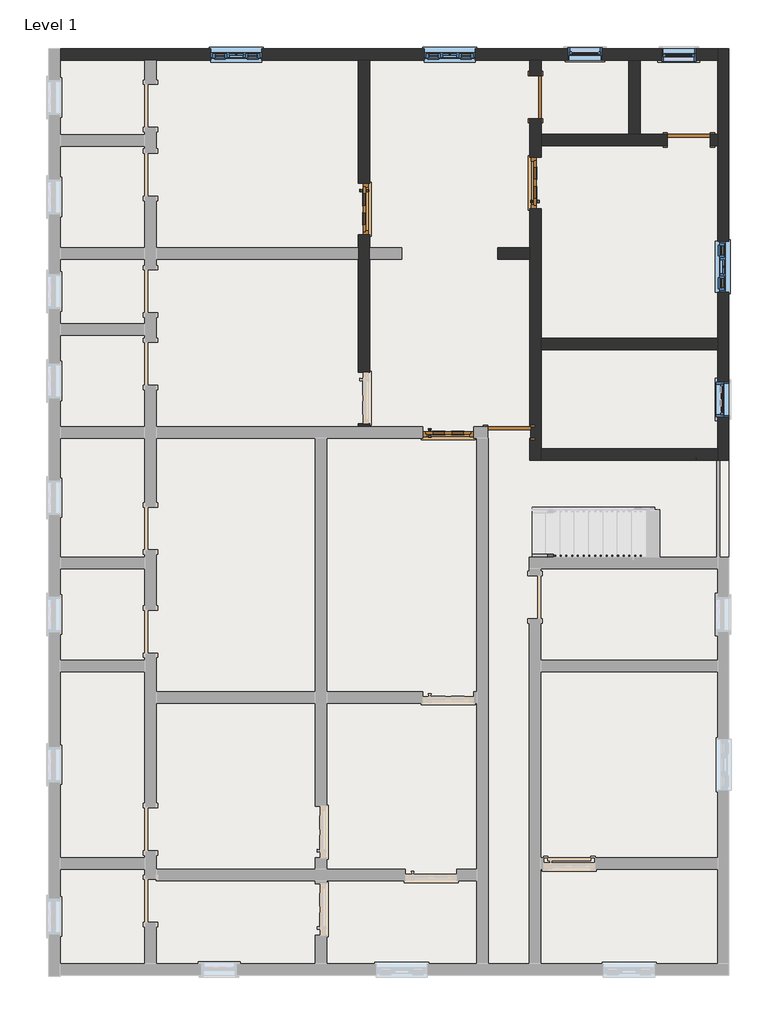
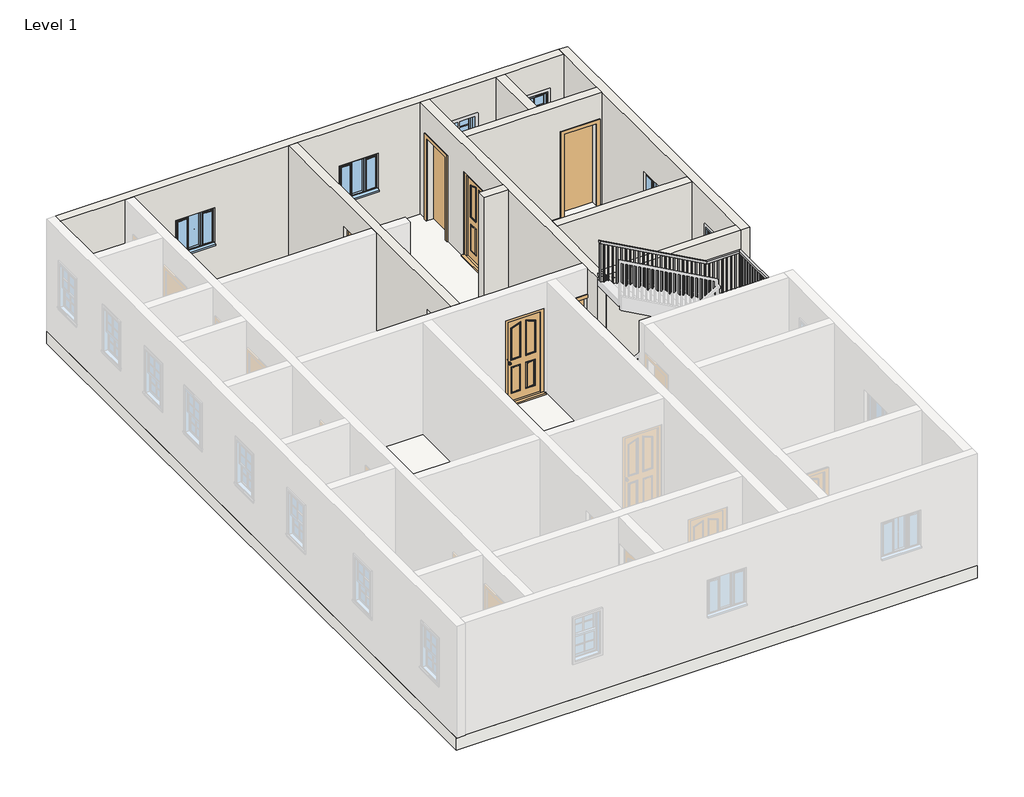
# One storey, part 2 of 3: 9 walls, 6 doors, 6 windows, 1 railing, 1 slab.
"""IFC4 building model written with IfcOpenShell, lengths in millimetres."""

from ifc_helpers import new_model, si_unit, frame, origin, origin_with_axes, place, context, project, spatial, polyline, outline, extrude, faceted_brep, transform, mapped, element, save
from components import doors_extsgl_12_910x2110mm_9a09825e, doors_extsgl_12_910x2110mm_ece77ece, door_fadea3f2, window_679d2811, windows_tpl_w_glazing_cross_bars_910x910mm_4aa0f884

model = new_model("IFC4")

# Units and contexts
model_context = context("Model", 3, world=origin())
ifc_project = project(units=[si_unit("LENGTHUNIT", "METRE", prefix="MILLI")], contexts=[model_context])

# Site, building, storey
site = spatial("IfcSite", under=ifc_project)
building = spatial("IfcBuilding", under=site)
storey = spatial("IfcBuildingStorey", under=building, Name="Level 1", Elevation=0.0)

# Doors
placement = place(None, origin())
doors_extsgl_12_910x2110mm_shape = doors_extsgl_12_910x2110mm_9a09825e(model_context)
element("IfcDoor", 1, ObjectType="Doors_ExtSgl_12 : 910x2110mm", at=placement, inside=storey, context=model_context, shape_type="MappedRepresentation", body=[
    mapped(doors_extsgl_12_910x2110mm_shape, transform((-4887.6876145, 4566.1404944, 0.0), x_axis=(0.0, -1.0, 0.0), y_axis=(1.0, 0.0, 0.0), z_axis=(0.0, 0.0, 1.0))),
])
element("IfcDoor", 2, ObjectType="Doors_ExtSgl_12 : 910x2110mm", at=placement, inside=storey, context=model_context, shape_type="MappedRepresentation", body=[
    mapped(doors_extsgl_12_910x2110mm_shape, transform((-1839.6876145, 5029.6904944, 0.0), x_axis=(0.0, 1.0, 0.0), y_axis=(-1.0, 0.0, 0.0), z_axis=(0.0, 0.0, 1.0))),
])
doors_extsgl_12_910x2110mm_2_shape = doors_extsgl_12_910x2110mm_ece77ece(model_context)
element("IfcDoor", 3, ObjectType="Doors_ExtSgl_12 : 910x2110mm", at=placement, inside=storey, context=model_context, shape_type="MappedRepresentation", body=[
    mapped(doors_extsgl_12_910x2110mm_2_shape, transform((-3389.0876145, 603.7404944, 0.0), x_axis=(1.0, 0.0, 0.0), y_axis=(0.0, 1.0, 0.0), z_axis=(0.0, 0.0, 1.0))),
])
door_shape = door_fadea3f2(model_context)
element("IfcDoor", 4, ObjectType="Single-Flush : 30\" x 80\"", at=placement, inside=storey, context=model_context, shape_type="MappedRepresentation", body=[
    mapped(door_shape, transform((-1839.6876145, 6550.5154944, 0.0), x_axis=(0.0, -1.0, 0.0), y_axis=(1.0, 0.0, 0.0), z_axis=(0.0, 0.0, 1.0))),
])
element("IfcDoor", 5, ObjectType="Single-Flush : 30\" x 80\"", at=placement, inside=storey, context=model_context, shape_type="MappedRepresentation", body=[
    mapped(door_shape, transform((878.1123855, 5791.6904944, 0.0), x_axis=(1.0, 0.0, 0.0), y_axis=(0.0, 1.0, 0.0), z_axis=(0.0, 0.0, 1.0))),
])
element("IfcDoor", 6, ObjectType="Single-Flush : 30\" x 80\"", at=placement, inside=storey, context=model_context, shape_type="MappedRepresentation", body=[
    mapped(door_shape, transform((-2309.5876145, 603.7404944, 0.0), x_axis=(1.0, 0.0, 0.0), y_axis=(0.0, 1.0, 0.0), z_axis=(0.0, 0.0, 1.0))),
])

# Railing
element("IfcRailing", 7, ObjectType="Handrail - Rectangular", at=placement, inside=storey, context=model_context, shape_type="SolidModel", body=[
    faceted_brep([(-1903.1876145, -1555.2595056, 1051.56), (-1903.1876145, -1555.2595056, 993.4879132), (-1903.1876145, -1606.0595056, 993.4879132), (-1903.1876145, -1606.0595056, 1051.56), (325.4830625, -1555.2595056, 2286.0), (338.6121628, -1555.2595056, 2235.2), (338.6121628, -1606.0595056, 2235.2), (325.4830625, -1606.0595056, 2286.0), (1322.6123855, -1555.2595056, 2286.0), (1322.6123855, -1555.2595056, 2235.2), (1373.4123855, -1606.0595056, 2235.2), (1373.4123855, -1606.0595056, 2286.0), (1322.6123855, 57.6404944, 2286.0), (1322.6123855, 57.6404944, 2235.2), (1373.4123855, 108.4404944, 2235.2), (1373.4123855, 108.4404944, 2286.0), (573.1131377, 57.6404944, 2286.0), (559.9840375, 57.6404944, 2235.2), (559.9840375, 108.4404944, 2235.2), (573.1131377, 108.4404944, 2286.0), (-1903.1876145, 57.6404944, 3657.6), (-1903.1876145, 108.4404944, 3657.6), (-1903.1876145, 108.4404944, 3599.5279132), (-1903.1876145, 57.6404944, 3599.5279132)], [[[0, 1, 2, 3]], [[1, 0, 4, 5]], [[2, 1, 5, 6]], [[3, 2, 6, 7]], [[0, 3, 7, 4]], [[5, 4, 8, 9]], [[6, 5, 9, 10]], [[7, 6, 10, 11]], [[4, 7, 11, 8]], [[9, 8, 12, 13]], [[10, 9, 13, 14]], [[11, 10, 14, 15]], [[8, 11, 15, 12]], [[13, 12, 16, 17]], [[14, 13, 17, 18]], [[15, 14, 18, 19]], [[12, 15, 19, 16]], [[20, 21, 22, 23]], [[17, 16, 20, 23]], [[18, 17, 23, 22]], [[19, 18, 22, 21]], [[16, 19, 21, 20]]]),
    extrude(outline(polyline([(3537.9768073, -1792.0626145), (3548.5284254, -1811.1126145), (2606.04, -1811.1126145), (2606.04, -1792.0626145), (3537.9768073, -1792.0626145)])), frame((0.0, 73.5154944, 0.0), z_axis=(0.0, 1.0, 0.0), x_axis=(0.0, 0.0, 1.0)), (0.0, 0.0, 1.0), 19.05),
    extrude(outline(polyline([(3481.7015104, -1690.4626145), (3492.2531286, -1709.5126145), (2606.04, -1709.5126145), (2606.04, -1690.4626145), (3481.7015104, -1690.4626145)])), frame((0.0, 73.5154944, 0.0), z_axis=(0.0, 1.0, 0.0), x_axis=(0.0, 0.0, 1.0)), (0.0, 0.0, 1.0), 19.05),
    extrude(outline(polyline([(3425.4262135, -1588.8626145), (3435.9778317, -1607.9126145), (2468.88, -1607.9126145), (2468.88, -1588.8626145), (3425.4262135, -1588.8626145)])), frame((0.0, 73.5154944, 0.0), z_axis=(0.0, 1.0, 0.0), x_axis=(0.0, 0.0, 1.0)), (0.0, 0.0, 1.0), 19.05),
    extrude(outline(polyline([(3369.1509166, -1487.2626145), (3379.7025348, -1506.3126145), (2468.88, -1506.3126145), (2468.88, -1487.2626145), (3369.1509166, -1487.2626145)])), frame((0.0, 73.5154944, 0.0), z_axis=(0.0, 1.0, 0.0), x_axis=(0.0, 0.0, 1.0)), (0.0, 0.0, 1.0), 19.05),
    extrude(outline(polyline([(3312.8756198, -1385.6626145), (3323.4272379, -1404.7126145), (2331.72, -1404.7126145), (2331.72, -1385.6626145), (3312.8756198, -1385.6626145)])), frame((0.0, 73.5154944, 0.0), z_axis=(0.0, 1.0, 0.0), x_axis=(0.0, 0.0, 1.0)), (0.0, 0.0, 1.0), 19.05),
    extrude(outline(polyline([(3256.6003229, -1284.0626145), (3267.151941, -1303.1126145), (2331.72, -1303.1126145), (2331.72, -1284.0626145), (3256.6003229, -1284.0626145)])), frame((0.0, 73.5154944, 0.0), z_axis=(0.0, 1.0, 0.0), x_axis=(0.0, 0.0, 1.0)), (0.0, 0.0, 1.0), 19.05),
    extrude(outline(polyline([(3200.325026, -1182.4626145), (3210.8766442, -1201.5126145), (2331.72, -1201.5126145), (2331.72, -1182.4626145), (3200.325026, -1182.4626145)])), frame((0.0, 73.5154944, 0.0), z_axis=(0.0, 1.0, 0.0), x_axis=(0.0, 0.0, 1.0)), (0.0, 0.0, 1.0), 19.05),
    extrude(outline(polyline([(3144.0497291, -1080.8626145), (3154.6013473, -1099.9126145), (2194.56, -1099.9126145), (2194.56, -1080.8626145), (3144.0497291, -1080.8626145)])), frame((0.0, 73.5154944, 0.0), z_axis=(0.0, 1.0, 0.0), x_axis=(0.0, 0.0, 1.0)), (0.0, 0.0, 1.0), 19.05),
    extrude(outline(polyline([(3087.7744322, -979.2626145), (3098.3260504, -998.3126145), (2194.56, -998.3126145), (2194.56, -979.2626145), (3087.7744322, -979.2626145)])), frame((0.0, 73.5154944, 0.0), z_axis=(0.0, 1.0, 0.0), x_axis=(0.0, 0.0, 1.0)), (0.0, 0.0, 1.0), 19.05),
    extrude(outline(polyline([(3031.4991354, -877.6626145), (3042.0507535, -896.7126145), (2057.4, -896.7126145), (2057.4, -877.6626145), (3031.4991354, -877.6626145)])), frame((0.0, 73.5154944, 0.0), z_axis=(0.0, 1.0, 0.0), x_axis=(0.0, 0.0, 1.0)), (0.0, 0.0, 1.0), 19.05),
    extrude(outline(polyline([(2975.2238385, -776.0626145), (2985.7754566, -795.1126145), (2057.4, -795.1126145), (2057.4, -776.0626145), (2975.2238385, -776.0626145)])), frame((0.0, 73.5154944, 0.0), z_axis=(0.0, 1.0, 0.0), x_axis=(0.0, 0.0, 1.0)), (0.0, 0.0, 1.0), 19.05),
    extrude(outline(polyline([(2918.9485416, -674.4626145), (2929.5001598, -693.5126145), (2057.4, -693.5126145), (2057.4, -674.4626145), (2918.9485416, -674.4626145)])), frame((0.0, 73.5154944, 0.0), z_axis=(0.0, 1.0, 0.0), x_axis=(0.0, 0.0, 1.0)), (0.0, 0.0, 1.0), 19.05),
    extrude(outline(polyline([(2862.6732447, -572.8626145), (2873.2248629, -591.9126145), (1920.24, -591.9126145), (1920.24, -572.8626145), (2862.6732447, -572.8626145)])), frame((0.0, 73.5154944, 0.0), z_axis=(0.0, 1.0, 0.0), x_axis=(0.0, 0.0, 1.0)), (0.0, 0.0, 1.0), 19.05),
    extrude(outline(polyline([(2806.3979478, -471.2626145), (2816.949566, -490.3126145), (1920.24, -490.3126145), (1920.24, -471.2626145), (2806.3979478, -471.2626145)])), frame((0.0, 73.5154944, 0.0), z_axis=(0.0, 1.0, 0.0), x_axis=(0.0, 0.0, 1.0)), (0.0, 0.0, 1.0), 19.05),
    extrude(outline(polyline([(2750.1226509, -369.6626145), (2760.6742691, -388.7126145), (1783.08, -388.7126145), (1783.08, -369.6626145), (2750.1226509, -369.6626145)])), frame((0.0, 73.5154944, 0.0), z_axis=(0.0, 1.0, 0.0), x_axis=(0.0, 0.0, 1.0)), (0.0, 0.0, 1.0), 19.05),
    extrude(outline(polyline([(2693.8473541, -268.0626145), (2704.3989722, -287.1126145), (1783.08, -287.1126145), (1783.08, -268.0626145), (2693.8473541, -268.0626145)])), frame((0.0, 73.5154944, 0.0), z_axis=(0.0, 1.0, 0.0), x_axis=(0.0, 0.0, 1.0)), (0.0, 0.0, 1.0), 19.05),
    extrude(outline(polyline([(2637.5720572, -166.4626145), (2648.1236754, -185.5126145), (1783.08, -185.5126145), (1783.08, -166.4626145), (2637.5720572, -166.4626145)])), frame((0.0, 73.5154944, 0.0), z_axis=(0.0, 1.0, 0.0), x_axis=(0.0, 0.0, 1.0)), (0.0, 0.0, 1.0), 19.05),
    extrude(outline(polyline([(2581.2967603, -64.8626145), (2591.8483785, -83.9126145), (1645.92, -83.9126145), (1645.92, -64.8626145), (2581.2967603, -64.8626145)])), frame((0.0, 73.5154944, 0.0), z_axis=(0.0, 1.0, 0.0), x_axis=(0.0, 0.0, 1.0)), (0.0, 0.0, 1.0), 19.05),
    extrude(outline(polyline([(2525.0214634, 36.7373855), (2535.5730816, 17.6873855), (1645.92, 17.6873855), (1645.92, 36.7373855), (2525.0214634, 36.7373855)])), frame((0.0, 73.5154944, 0.0), z_axis=(0.0, 1.0, 0.0), x_axis=(0.0, 0.0, 1.0)), (0.0, 0.0, 1.0), 19.05),
    extrude(outline(polyline([(2468.7461665, 138.3373855), (2479.2977847, 119.2873855), (1508.76, 119.2873855), (1508.76, 138.3373855), (2468.7461665, 138.3373855)])), frame((0.0, 73.5154944, 0.0), z_axis=(0.0, 1.0, 0.0), x_axis=(0.0, 0.0, 1.0)), (0.0, 0.0, 1.0), 19.05),
    extrude(outline(polyline([(2412.4708697, 239.9373855), (2423.0224878, 220.8873855), (1508.76, 220.8873855), (1508.76, 239.9373855), (2412.4708697, 239.9373855)])), frame((0.0, 73.5154944, 0.0), z_axis=(0.0, 1.0, 0.0), x_axis=(0.0, 0.0, 1.0)), (0.0, 0.0, 1.0), 19.05),
    extrude(outline(polyline([(2356.1955728, 341.5373855), (2366.7471909, 322.4873855), (1371.6, 322.4873855), (1371.6, 341.5373855), (2356.1955728, 341.5373855)])), frame((0.0, 73.5154944, 0.0), z_axis=(0.0, 1.0, 0.0), x_axis=(0.0, 0.0, 1.0)), (0.0, 0.0, 1.0), 19.05),
    extrude(outline(polyline([(2299.9202759, 443.1373855), (2310.4718941, 424.0873855), (1371.6, 424.0873855), (1371.6, 443.1373855), (2299.9202759, 443.1373855)])), frame((0.0, 73.5154944, 0.0), z_axis=(0.0, 1.0, 0.0), x_axis=(0.0, 0.0, 1.0)), (0.0, 0.0, 1.0), 19.05),
    extrude(outline(polyline([(2243.644979, 544.7373855), (2254.1965972, 525.6873855), (1371.6, 525.6873855), (1371.6, 544.7373855), (2243.644979, 544.7373855)])), frame((0.0, 73.5154944, 0.0), z_axis=(0.0, 1.0, 0.0), x_axis=(0.0, 0.0, 1.0)), (0.0, 0.0, 1.0), 19.05),
    extrude(outline(polyline([(646.3373855, 92.5654944), (646.3373855, 73.5154944), (627.2873855, 73.5154944), (627.2873855, 92.5654944), (646.3373855, 92.5654944)])), frame((0.0, 0.0, 1371.6), z_axis=(0.0, 0.0, 1.0), x_axis=(1.0, 0.0, 0.0)), (0.0, 0.0, 1.0), 863.6),
    extrude(outline(polyline([(747.9373855, 92.5654944), (747.9373855, 73.5154944), (728.8873855, 73.5154944), (728.8873855, 92.5654944), (747.9373855, 92.5654944)])), frame((0.0, 0.0, 1371.6), z_axis=(0.0, 0.0, 1.0), x_axis=(1.0, 0.0, 0.0)), (0.0, 0.0, 1.0), 863.6),
    extrude(outline(polyline([(849.5373855, 92.5654944), (849.5373855, 73.5154944), (830.4873855, 73.5154944), (830.4873855, 92.5654944), (849.5373855, 92.5654944)])), frame((0.0, 0.0, 1371.6), z_axis=(0.0, 0.0, 1.0), x_axis=(1.0, 0.0, 0.0)), (0.0, 0.0, 1.0), 863.6),
    extrude(outline(polyline([(951.1373855, 92.5654944), (951.1373855, 73.5154944), (932.0873855, 73.5154944), (932.0873855, 92.5654944), (951.1373855, 92.5654944)])), frame((0.0, 0.0, 1371.6), z_axis=(0.0, 0.0, 1.0), x_axis=(1.0, 0.0, 0.0)), (0.0, 0.0, 1.0), 863.6),
    extrude(outline(polyline([(1052.7373855, 92.5654944), (1052.7373855, 73.5154944), (1033.6873855, 73.5154944), (1033.6873855, 92.5654944), (1052.7373855, 92.5654944)])), frame((0.0, 0.0, 1371.6), z_axis=(0.0, 0.0, 1.0), x_axis=(1.0, 0.0, 0.0)), (0.0, 0.0, 1.0), 863.6),
    extrude(outline(polyline([(1154.3373855, 92.5654944), (1154.3373855, 73.5154944), (1135.2873855, 73.5154944), (1135.2873855, 92.5654944), (1154.3373855, 92.5654944)])), frame((0.0, 0.0, 1371.6), z_axis=(0.0, 0.0, 1.0), x_axis=(1.0, 0.0, 0.0)), (0.0, 0.0, 1.0), 863.6),
    extrude(outline(polyline([(1255.9373855, 92.5654944), (1255.9373855, 73.5154944), (1236.8873855, 73.5154944), (1236.8873855, 92.5654944), (1255.9373855, 92.5654944)])), frame((0.0, 0.0, 1371.6), z_axis=(0.0, 0.0, 1.0), x_axis=(1.0, 0.0, 0.0)), (0.0, 0.0, 1.0), 863.6),
    extrude(outline(polyline([(1357.5373855, 35.4154944), (1338.4873855, 35.4154944), (1338.4873855, 54.4654944), (1357.5373855, 54.4654944), (1357.5373855, 35.4154944)])), frame((0.0, 0.0, 1371.6), z_axis=(0.0, 0.0, 1.0), x_axis=(1.0, 0.0, 0.0)), (0.0, 0.0, 1.0), 863.6),
    extrude(outline(polyline([(1357.5373855, -66.1845056), (1338.4873855, -66.1845056), (1338.4873855, -47.1345056), (1357.5373855, -47.1345056), (1357.5373855, -66.1845056)])), frame((0.0, 0.0, 1371.6), z_axis=(0.0, 0.0, 1.0), x_axis=(1.0, 0.0, 0.0)), (0.0, 0.0, 1.0), 863.6),
    extrude(outline(polyline([(1357.5373855, -167.7845056), (1338.4873855, -167.7845056), (1338.4873855, -148.7345056), (1357.5373855, -148.7345056), (1357.5373855, -167.7845056)])), frame((0.0, 0.0, 1371.6), z_axis=(0.0, 0.0, 1.0), x_axis=(1.0, 0.0, 0.0)), (0.0, 0.0, 1.0), 863.6),
    extrude(outline(polyline([(1357.5373855, -269.3845056), (1338.4873855, -269.3845056), (1338.4873855, -250.3345056), (1357.5373855, -250.3345056), (1357.5373855, -269.3845056)])), frame((0.0, 0.0, 1371.6), z_axis=(0.0, 0.0, 1.0), x_axis=(1.0, 0.0, 0.0)), (0.0, 0.0, 1.0), 863.6),
    extrude(outline(polyline([(1357.5373855, -370.9845056), (1338.4873855, -370.9845056), (1338.4873855, -351.9345056), (1357.5373855, -351.9345056), (1357.5373855, -370.9845056)])), frame((0.0, 0.0, 1371.6), z_axis=(0.0, 0.0, 1.0), x_axis=(1.0, 0.0, 0.0)), (0.0, 0.0, 1.0), 863.6),
    extrude(outline(polyline([(1357.5373855, -472.5845056), (1338.4873855, -472.5845056), (1338.4873855, -453.5345056), (1357.5373855, -453.5345056), (1357.5373855, -472.5845056)])), frame((0.0, 0.0, 1371.6), z_axis=(0.0, 0.0, 1.0), x_axis=(1.0, 0.0, 0.0)), (0.0, 0.0, 1.0), 863.6),
    extrude(outline(polyline([(1357.5373855, -574.1845056), (1338.4873855, -574.1845056), (1338.4873855, -555.1345056), (1357.5373855, -555.1345056), (1357.5373855, -574.1845056)])), frame((0.0, 0.0, 1371.6), z_axis=(0.0, 0.0, 1.0), x_axis=(1.0, 0.0, 0.0)), (0.0, 0.0, 1.0), 863.6),
    extrude(outline(polyline([(1357.5373855, -675.7845056), (1338.4873855, -675.7845056), (1338.4873855, -656.7345056), (1357.5373855, -656.7345056), (1357.5373855, -675.7845056)])), frame((0.0, 0.0, 1371.6), z_axis=(0.0, 0.0, 1.0), x_axis=(1.0, 0.0, 0.0)), (0.0, 0.0, 1.0), 863.6),
    extrude(outline(polyline([(1357.5373855, -777.3845056), (1338.4873855, -777.3845056), (1338.4873855, -758.3345056), (1357.5373855, -758.3345056), (1357.5373855, -777.3845056)])), frame((0.0, 0.0, 1371.6), z_axis=(0.0, 0.0, 1.0), x_axis=(1.0, 0.0, 0.0)), (0.0, 0.0, 1.0), 863.6),
    extrude(outline(polyline([(1357.5373855, -878.9845056), (1338.4873855, -878.9845056), (1338.4873855, -859.9345056), (1357.5373855, -859.9345056), (1357.5373855, -878.9845056)])), frame((0.0, 0.0, 1371.6), z_axis=(0.0, 0.0, 1.0), x_axis=(1.0, 0.0, 0.0)), (0.0, 0.0, 1.0), 863.6),
    extrude(outline(polyline([(1357.5373855, -980.5845056), (1338.4873855, -980.5845056), (1338.4873855, -961.5345056), (1357.5373855, -961.5345056), (1357.5373855, -980.5845056)])), frame((0.0, 0.0, 1371.6), z_axis=(0.0, 0.0, 1.0), x_axis=(1.0, 0.0, 0.0)), (0.0, 0.0, 1.0), 863.6),
    extrude(outline(polyline([(1357.5373855, -1082.1845056), (1338.4873855, -1082.1845056), (1338.4873855, -1063.1345056), (1357.5373855, -1063.1345056), (1357.5373855, -1082.1845056)])), frame((0.0, 0.0, 1371.6), z_axis=(0.0, 0.0, 1.0), x_axis=(1.0, 0.0, 0.0)), (0.0, 0.0, 1.0), 863.6),
    extrude(outline(polyline([(1357.5373855, -1183.7845056), (1338.4873855, -1183.7845056), (1338.4873855, -1164.7345056), (1357.5373855, -1164.7345056), (1357.5373855, -1183.7845056)])), frame((0.0, 0.0, 1371.6), z_axis=(0.0, 0.0, 1.0), x_axis=(1.0, 0.0, 0.0)), (0.0, 0.0, 1.0), 863.6),
    extrude(outline(polyline([(1357.5373855, -1285.3845056), (1338.4873855, -1285.3845056), (1338.4873855, -1266.3345056), (1357.5373855, -1266.3345056), (1357.5373855, -1285.3845056)])), frame((0.0, 0.0, 1371.6), z_axis=(0.0, 0.0, 1.0), x_axis=(1.0, 0.0, 0.0)), (0.0, 0.0, 1.0), 863.6),
    extrude(outline(polyline([(1357.5373855, -1386.9845056), (1338.4873855, -1386.9845056), (1338.4873855, -1367.9345056), (1357.5373855, -1367.9345056), (1357.5373855, -1386.9845056)])), frame((0.0, 0.0, 1371.6), z_axis=(0.0, 0.0, 1.0), x_axis=(1.0, 0.0, 0.0)), (0.0, 0.0, 1.0), 863.6),
    extrude(outline(polyline([(1357.5373855, -1488.5845056), (1338.4873855, -1488.5845056), (1338.4873855, -1469.5345056), (1357.5373855, -1469.5345056), (1357.5373855, -1488.5845056)])), frame((0.0, 0.0, 1371.6), z_axis=(0.0, 0.0, 1.0), x_axis=(1.0, 0.0, 0.0)), (0.0, 0.0, 1.0), 863.6),
    extrude(outline(polyline([(1236.8873855, -1590.1845056), (1236.8873855, -1571.1345056), (1255.9373855, -1571.1345056), (1255.9373855, -1590.1845056), (1236.8873855, -1590.1845056)])), frame((0.0, 0.0, 1371.6), z_axis=(0.0, 0.0, 1.0), x_axis=(1.0, 0.0, 0.0)), (0.0, 0.0, 1.0), 863.6),
    extrude(outline(polyline([(1135.2873855, -1590.1845056), (1135.2873855, -1571.1345056), (1154.3373855, -1571.1345056), (1154.3373855, -1590.1845056), (1135.2873855, -1590.1845056)])), frame((0.0, 0.0, 1371.6), z_axis=(0.0, 0.0, 1.0), x_axis=(1.0, 0.0, 0.0)), (0.0, 0.0, 1.0), 863.6),
    extrude(outline(polyline([(1033.6873855, -1590.1845056), (1033.6873855, -1571.1345056), (1052.7373855, -1571.1345056), (1052.7373855, -1590.1845056), (1033.6873855, -1590.1845056)])), frame((0.0, 0.0, 1371.6), z_axis=(0.0, 0.0, 1.0), x_axis=(1.0, 0.0, 0.0)), (0.0, 0.0, 1.0), 863.6),
    extrude(outline(polyline([(932.0873855, -1590.1845056), (932.0873855, -1571.1345056), (951.1373855, -1571.1345056), (951.1373855, -1590.1845056), (932.0873855, -1590.1845056)])), frame((0.0, 0.0, 1371.6), z_axis=(0.0, 0.0, 1.0), x_axis=(1.0, 0.0, 0.0)), (0.0, 0.0, 1.0), 863.6),
    extrude(outline(polyline([(830.4873855, -1590.1845056), (830.4873855, -1571.1345056), (849.5373855, -1571.1345056), (849.5373855, -1590.1845056), (830.4873855, -1590.1845056)])), frame((0.0, 0.0, 1371.6), z_axis=(0.0, 0.0, 1.0), x_axis=(1.0, 0.0, 0.0)), (0.0, 0.0, 1.0), 863.6),
    extrude(outline(polyline([(728.8873855, -1590.1845056), (728.8873855, -1571.1345056), (747.9373855, -1571.1345056), (747.9373855, -1590.1845056), (728.8873855, -1590.1845056)])), frame((0.0, 0.0, 1371.6), z_axis=(0.0, 0.0, 1.0), x_axis=(1.0, 0.0, 0.0)), (0.0, 0.0, 1.0), 863.6),
    extrude(outline(polyline([(627.2873855, -1590.1845056), (627.2873855, -1571.1345056), (646.3373855, -1571.1345056), (646.3373855, -1590.1845056), (627.2873855, -1590.1845056)])), frame((0.0, 0.0, 1371.6), z_axis=(0.0, 0.0, 1.0), x_axis=(1.0, 0.0, 0.0)), (0.0, 0.0, 1.0), 863.6),
    extrude(outline(polyline([(525.6873855, -1590.1845056), (525.6873855, -1571.1345056), (544.7373855, -1571.1345056), (544.7373855, -1590.1845056), (525.6873855, -1590.1845056)])), frame((0.0, 0.0, 1371.6), z_axis=(0.0, 0.0, 1.0), x_axis=(1.0, 0.0, 0.0)), (0.0, 0.0, 1.0), 863.6),
    extrude(outline(polyline([(424.0873855, -1590.1845056), (424.0873855, -1571.1345056), (443.1373855, -1571.1345056), (443.1373855, -1590.1845056), (424.0873855, -1590.1845056)])), frame((0.0, 0.0, 1371.6), z_axis=(0.0, 0.0, 1.0), x_axis=(1.0, 0.0, 0.0)), (0.0, 0.0, 1.0), 863.6),
    extrude(outline(polyline([(322.4873855, -1590.1845056), (322.4873855, -1571.1345056), (341.5373855, -1571.1345056), (341.5373855, -1590.1845056), (322.4873855, -1590.1845056)])), frame((0.0, 0.0, 1371.6), z_axis=(0.0, 0.0, 1.0), x_axis=(1.0, 0.0, 0.0)), (0.0, 0.0, 1.0), 863.6),
    extrude(outline(polyline([(2180.5449568, 239.9373855), (2169.9933387, 220.8873855), (1234.44, 220.8873855), (1234.44, 239.9373855), (2180.5449568, 239.9373855)])), frame((0.0, -1590.1845056, 0.0), z_axis=(0.0, 1.0, 0.0), x_axis=(0.0, 0.0, 1.0)), (0.0, 0.0, 1.0), 19.05),
    extrude(outline(polyline([(2124.26966, 138.3373855), (2113.7180418, 119.2873855), (1234.44, 119.2873855), (1234.44, 138.3373855), (2124.26966, 138.3373855)])), frame((0.0, -1590.1845056, 0.0), z_axis=(0.0, 1.0, 0.0), x_axis=(0.0, 0.0, 1.0)), (0.0, 0.0, 1.0), 19.05),
    extrude(outline(polyline([(2067.9943631, 36.7373855), (2057.4427449, 17.6873855), (1097.28, 17.6873855), (1097.28, 36.7373855), (2067.9943631, 36.7373855)])), frame((0.0, -1590.1845056, 0.0), z_axis=(0.0, 1.0, 0.0), x_axis=(0.0, 0.0, 1.0)), (0.0, 0.0, 1.0), 19.05),
    extrude(outline(polyline([(2011.7190662, -64.8626145), (2001.167448, -83.9126145), (1097.28, -83.9126145), (1097.28, -64.8626145), (2011.7190662, -64.8626145)])), frame((0.0, -1590.1845056, 0.0), z_axis=(0.0, 1.0, 0.0), x_axis=(0.0, 0.0, 1.0)), (0.0, 0.0, 1.0), 19.05),
    extrude(outline(polyline([(1955.4437693, -166.4626145), (1944.8921511, -185.5126145), (960.12, -185.5126145), (960.12, -166.4626145), (1955.4437693, -166.4626145)])), frame((0.0, -1590.1845056, 0.0), z_axis=(0.0, 1.0, 0.0), x_axis=(0.0, 0.0, 1.0)), (0.0, 0.0, 1.0), 19.05),
    extrude(outline(polyline([(1899.1684724, -268.0626145), (1888.6168543, -287.1126145), (960.12, -287.1126145), (960.12, -268.0626145), (1899.1684724, -268.0626145)])), frame((0.0, -1590.1845056, 0.0), z_axis=(0.0, 1.0, 0.0), x_axis=(0.0, 0.0, 1.0)), (0.0, 0.0, 1.0), 19.05),
    extrude(outline(polyline([(1842.8931755, -369.6626145), (1832.3415574, -388.7126145), (960.12, -388.7126145), (960.12, -369.6626145), (1842.8931755, -369.6626145)])), frame((0.0, -1590.1845056, 0.0), z_axis=(0.0, 1.0, 0.0), x_axis=(0.0, 0.0, 1.0)), (0.0, 0.0, 1.0), 19.05),
    extrude(outline(polyline([(1786.6178787, -471.2626145), (1776.0662605, -490.3126145), (822.96, -490.3126145), (822.96, -471.2626145), (1786.6178787, -471.2626145)])), frame((0.0, -1590.1845056, 0.0), z_axis=(0.0, 1.0, 0.0), x_axis=(0.0, 0.0, 1.0)), (0.0, 0.0, 1.0), 19.05),
    extrude(outline(polyline([(1730.3425818, -572.8626145), (1719.7909636, -591.9126145), (822.96, -591.9126145), (822.96, -572.8626145), (1730.3425818, -572.8626145)])), frame((0.0, -1590.1845056, 0.0), z_axis=(0.0, 1.0, 0.0), x_axis=(0.0, 0.0, 1.0)), (0.0, 0.0, 1.0), 19.05),
    extrude(outline(polyline([(1674.0672849, -674.4626145), (1663.5156667, -693.5126145), (685.8, -693.5126145), (685.8, -674.4626145), (1674.0672849, -674.4626145)])), frame((0.0, -1590.1845056, 0.0), z_axis=(0.0, 1.0, 0.0), x_axis=(0.0, 0.0, 1.0)), (0.0, 0.0, 1.0), 19.05),
    extrude(outline(polyline([(1617.791988, -776.0626145), (1607.2403699, -795.1126145), (685.8, -795.1126145), (685.8, -776.0626145), (1617.791988, -776.0626145)])), frame((0.0, -1590.1845056, 0.0), z_axis=(0.0, 1.0, 0.0), x_axis=(0.0, 0.0, 1.0)), (0.0, 0.0, 1.0), 19.05),
    extrude(outline(polyline([(1561.5166911, -877.6626145), (1550.965073, -896.7126145), (685.8, -896.7126145), (685.8, -877.6626145), (1561.5166911, -877.6626145)])), frame((0.0, -1590.1845056, 0.0), z_axis=(0.0, 1.0, 0.0), x_axis=(0.0, 0.0, 1.0)), (0.0, 0.0, 1.0), 19.05),
    extrude(outline(polyline([(1505.2413943, -979.2626145), (1494.6897761, -998.3126145), (548.64, -998.3126145), (548.64, -979.2626145), (1505.2413943, -979.2626145)])), frame((0.0, -1590.1845056, 0.0), z_axis=(0.0, 1.0, 0.0), x_axis=(0.0, 0.0, 1.0)), (0.0, 0.0, 1.0), 19.05),
    extrude(outline(polyline([(1448.9660974, -1080.8626145), (1438.4144792, -1099.9126145), (548.64, -1099.9126145), (548.64, -1080.8626145), (1448.9660974, -1080.8626145)])), frame((0.0, -1590.1845056, 0.0), z_axis=(0.0, 1.0, 0.0), x_axis=(0.0, 0.0, 1.0)), (0.0, 0.0, 1.0), 19.05),
    extrude(outline(polyline([(1392.6908005, -1182.4626145), (1382.1391823, -1201.5126145), (411.48, -1201.5126145), (411.48, -1182.4626145), (1392.6908005, -1182.4626145)])), frame((0.0, -1590.1845056, 0.0), z_axis=(0.0, 1.0, 0.0), x_axis=(0.0, 0.0, 1.0)), (0.0, 0.0, 1.0), 19.05),
    extrude(outline(polyline([(1336.4155036, -1284.0626145), (1325.8638855, -1303.1126145), (411.48, -1303.1126145), (411.48, -1284.0626145), (1336.4155036, -1284.0626145)])), frame((0.0, -1590.1845056, 0.0), z_axis=(0.0, 1.0, 0.0), x_axis=(0.0, 0.0, 1.0)), (0.0, 0.0, 1.0), 19.05),
    extrude(outline(polyline([(1280.1402067, -1385.6626145), (1269.5885886, -1404.7126145), (411.48, -1404.7126145), (411.48, -1385.6626145), (1280.1402067, -1385.6626145)])), frame((0.0, -1590.1845056, 0.0), z_axis=(0.0, 1.0, 0.0), x_axis=(0.0, 0.0, 1.0)), (0.0, 0.0, 1.0), 19.05),
    extrude(outline(polyline([(1223.8649099, -1487.2626145), (1213.3132917, -1506.3126145), (274.32, -1506.3126145), (274.32, -1487.2626145), (1223.8649099, -1487.2626145)])), frame((0.0, -1590.1845056, 0.0), z_axis=(0.0, 1.0, 0.0), x_axis=(0.0, 0.0, 1.0)), (0.0, 0.0, 1.0), 19.05),
    extrude(outline(polyline([(1167.589613, -1588.8626145), (1157.0379948, -1607.9126145), (274.32, -1607.9126145), (274.32, -1588.8626145), (1167.589613, -1588.8626145)])), frame((0.0, -1590.1845056, 0.0), z_axis=(0.0, 1.0, 0.0), x_axis=(0.0, 0.0, 1.0)), (0.0, 0.0, 1.0), 19.05),
    extrude(outline(polyline([(1111.3143161, -1690.4626145), (1100.7626979, -1709.5126145), (137.16, -1709.5126145), (137.16, -1690.4626145), (1111.3143161, -1690.4626145)])), frame((0.0, -1590.1845056, 0.0), z_axis=(0.0, 1.0, 0.0), x_axis=(0.0, 0.0, 1.0)), (0.0, 0.0, 1.0), 19.05),
    extrude(outline(polyline([(1055.0390192, -1792.0626145), (1044.487401, -1811.1126145), (137.16, -1811.1126145), (137.16, -1792.0626145), (1055.0390192, -1792.0626145)])), frame((0.0, -1590.1845056, 0.0), z_axis=(0.0, 1.0, 0.0), x_axis=(0.0, 0.0, 1.0)), (0.0, 0.0, 1.0), 19.05),
    extrude(outline(polyline([(1357.5373855, 73.5154944), (1338.4873855, 73.5154944), (1338.4873855, 92.5654944), (1357.5373855, 92.5654944), (1357.5373855, 73.5154944)])), frame((0.0, 0.0, 1371.6), z_axis=(0.0, 0.0, 1.0), x_axis=(1.0, 0.0, 0.0)), (0.0, 0.0, 1.0), 863.6),
    extrude(outline(polyline([(1338.4873855, -1590.1845056), (1338.4873855, -1571.1345056), (1357.5373855, -1571.1345056), (1357.5373855, -1590.1845056), (1338.4873855, -1590.1845056)])), frame((0.0, 0.0, 1371.6), z_axis=(0.0, 0.0, 1.0), x_axis=(1.0, 0.0, 0.0)), (0.0, 0.0, 1.0), 863.6),
    extrude(outline(polyline([(3588.9762951, -1884.1376145), (3599.5279132, -1903.1876145), (2606.04, -1903.1876145), (2606.04, -1884.1376145), (3588.9762951, -1884.1376145)])), frame((0.0, 73.5154944, 0.0), z_axis=(0.0, 1.0, 0.0), x_axis=(0.0, 0.0, 1.0)), (0.0, 0.0, 1.0), 19.05),
    extrude(outline(polyline([(1004.0395314, -1884.1376145), (993.4879132, -1903.1876145), (137.16, -1903.1876145), (137.16, -1884.1376145), (1004.0395314, -1884.1376145)])), frame((0.0, -1590.1845056, 0.0), z_axis=(0.0, 1.0, 0.0), x_axis=(0.0, 0.0, 1.0)), (0.0, 0.0, 1.0), 19.05),
])

# Slab
element("IfcSlab", 8, ObjectType="Generic - 12\"", at=placement, inside=storey, context=model_context, shape_type="SweptSolid", body=[
    extrude(outline(polyline([(1589.3123855, 7410.9404944), (1589.3123855, -9022.8595056), (-10475.6876145, -9022.8595056), (-10475.6876145, 7410.9404944), (1589.3123855, 7410.9404944)])), frame((0.0, 0.0, -304.8), z_axis=(0.0, 0.0, 1.0), x_axis=(1.0, 0.0, 0.0)), (0.0, 0.0, 1.0), 304.8),
])

# Walls
element("IfcWall", 9, ObjectType="4.5\"", at=placement, inside=storey, context=model_context, shape_type="Brep", body=[
    faceted_brep([(-4989.2876145, 758.3404944, 2110.0), (-4989.2876145, 758.3404944, 0.0), (-4989.2876145, 705.3404944, 0.0), (-4989.2876145, 705.3404944, 2743.2), (-4989.2876145, 3677.1404944, 2743.2), (-4989.2876145, 3880.3404944, 2743.2), (-4989.2876145, 7207.7404944, 2743.2), (-4989.2876145, 7207.7404944, 0.0), (-4989.2876145, 5021.1404944, 0.0), (-4989.2876145, 5021.1404944, 2110.0), (-4989.2876145, 4111.1404944, 2110.0), (-4989.2876145, 4111.1404944, 0.0), (-4989.2876145, 3880.3404944, 0.0), (-4989.2876145, 3677.1404944, 0.0), (-4989.2876145, 1668.3404944, 0.0), (-4989.2876145, 1668.3404944, 2110.0), (-4786.0876145, 705.3404944, 0.0), (-4786.0876145, 758.3404944, 0.0), (-4786.0876145, 758.3404944, 2110.0), (-4786.0876145, 1668.3404944, 2110.0), (-4786.0876145, 1668.3404944, 0.0), (-4786.0876145, 3677.1404944, 0.0), (-4786.0876145, 3880.3404944, 0.0), (-4786.0876145, 4111.1404944, 0.0), (-4786.0876145, 4111.1404944, 2110.0), (-4786.0876145, 5021.1404944, 2110.0), (-4786.0876145, 5021.1404944, 0.0), (-4786.0876145, 7207.7404944, 0.0), (-4786.0876145, 7207.7404944, 2743.2), (-4786.0876145, 3880.3404944, 2743.2), (-4786.0876145, 3677.1404944, 2743.2), (-4786.0876145, 705.3404944, 2743.2)], [[[0, 1, 2, 3, 4, 5, 6, 7, 8, 9, 10, 11, 12, 13, 14, 15]], [[16, 17, 18, 19, 20, 21, 22, 23, 24, 25, 26, 27, 28, 29, 30, 31]], [[8, 7, 27, 26]], [[2, 1, 17, 16]], [[14, 13, 12, 11, 23, 22, 21, 20]], [[7, 6, 28, 27]], [[3, 2, 16, 31]], [[26, 25, 9, 8]], [[24, 23, 11, 10]], [[25, 24, 10, 9]], [[20, 19, 15, 14]], [[18, 17, 1, 0]], [[19, 18, 0, 15]], [[6, 5, 4, 3, 31, 30, 29, 28]]]),
])
element("IfcWall", 10, ObjectType="4.5\"", at=placement, inside=storey, context=model_context, shape_type="Brep", body=[
    faceted_brep([(-1941.2876145, 6169.5154944, 0.0), (-1941.2876145, 5484.6904944, 0.0), (-1941.2876145, 5484.6904944, 2110.0), (-1941.2876145, 4574.6904944, 2110.0), (-1941.2876145, 4574.6904944, 0.0), (-1941.2876145, 3880.3404944, 0.0), (-1941.2876145, 3677.1404944, 0.0), (-1941.2876145, 705.3404944, 0.0), (-1941.2876145, 705.3404944, 2032.0), (-1941.2876145, 502.1404944, 2032.0), (-1941.2876145, 502.1404944, 0.0), (-1941.2876145, 108.4404944, 0.0), (-1941.2876145, 108.4404944, 2743.2), (-1941.2876145, 502.1404944, 2743.2), (-1941.2876145, 705.3404944, 2743.2), (-1941.2876145, 3677.1404944, 2743.2), (-1941.2876145, 3880.3404944, 2743.2), (-1941.2876145, 7207.7404944, 2743.2), (-1941.2876145, 7207.7404944, 0.0), (-1941.2876145, 6931.5154944, 0.0), (-1941.2876145, 6931.5154944, 2032.0), (-1941.2876145, 6169.5154944, 2032.0), (-1738.0876145, 5484.6904944, 2110.0), (-1738.0876145, 5484.6904944, 0.0), (-1738.0876145, 5690.0904944, 0.0), (-1738.0876145, 5893.2904944, 0.0), (-1738.0876145, 6169.5154944, 0.0), (-1738.0876145, 6169.5154944, 2032.0), (-1738.0876145, 6931.5154944, 2032.0), (-1738.0876145, 6931.5154944, 0.0), (-1738.0876145, 7207.7404944, 0.0), (-1738.0876145, 7207.7404944, 2743.2), (-1738.0876145, 5893.2904944, 2743.2), (-1738.0876145, 5690.0904944, 2743.2), (-1738.0876145, 2272.4885783, 2743.2), (-1738.0876145, 2069.2885783, 2743.2), (-1738.0876145, 311.6404944, 2743.2), (-1738.0876145, 108.4404944, 2743.2), (-1738.0876145, 108.4404944, 0.0), (-1738.0876145, 311.6404944, 0.0), (-1738.0876145, 2069.2885783, 0.0), (-1738.0876145, 2272.4885783, 0.0), (-1738.0876145, 4574.6904944, 0.0), (-1738.0876145, 4574.6904944, 2110.0), (-1928.5876145, 502.1404944, 0.0), (-1928.5876145, 705.3404944, 0.0), (-1928.5876145, 502.1404944, 2032.0), (-1928.5876145, 705.3404944, 2032.0)], [[[0, 1, 2, 3, 4, 5, 6, 7, 8, 9, 10, 11, 12, 13, 14, 15, 16, 17, 18, 19, 20, 21]], [[22, 23, 24, 25, 26, 27, 28, 29, 30, 31, 32, 33, 34, 35, 36, 37, 38, 39, 40, 41, 42, 43]], [[18, 30, 29, 19]], [[42, 41, 40, 39, 38, 11, 10, 44, 45, 7, 6, 5, 4]], [[26, 25, 24, 23, 1, 0]], [[18, 17, 31, 30]], [[12, 11, 38, 37]], [[27, 26, 0, 21]], [[28, 27, 21, 20]], [[29, 28, 20, 19]], [[46, 44, 10, 9]], [[45, 47, 8, 7]], [[44, 46, 47, 45]], [[47, 46, 9, 8]], [[4, 3, 43, 42]], [[2, 1, 23, 22]], [[3, 2, 22, 43]], [[17, 16, 15, 14, 13, 12, 37, 36, 35, 34, 33, 32, 31]]]),
])
element("IfcWall", 11, ObjectType="4.5\"", at=placement, inside=storey, context=model_context, shape_type="SweptSolid", body=[
    extrude(outline(polyline([(-2512.7876145, 3880.3404944), (-1941.2876145, 3880.3404944), (-1941.2876145, 3677.1404944), (-2512.7876145, 3677.1404944), (-2512.7876145, 3880.3404944)])), origin_with_axes(), (0.0, 0.0, 1.0), 2743.2),
])
element("IfcWall", 12, ObjectType="4.5\"", at=placement, inside=storey, context=model_context, shape_type="SweptSolid", body=[
    extrude(outline(polyline([(1386.1123855, 108.4404944), (-1738.0876145, 108.4404944), (-1738.0876145, 311.6404944), (1386.1123855, 311.6404944), (1386.1123855, 108.4404944)])), origin_with_axes(), (0.0, 0.0, 1.0), 2743.2),
])
element("IfcWall", 13, ObjectType="4.5\"", at=placement, inside=storey, context=model_context, shape_type="SweptSolid", body=[
    extrude(outline(polyline([(1386.1123855, 2069.2885783), (-1738.0876145, 2069.2885783), (-1738.0876145, 2272.4885783), (1386.1123855, 2272.4885783), (1386.1123855, 2069.2885783)])), origin_with_axes(), (0.0, 0.0, 1.0), 2743.2),
])
element("IfcWall", 14, ObjectType="4.5\"", at=placement, inside=storey, context=model_context, shape_type="Brep", body=[
    faceted_brep([(1259.1123855, 5690.0904944, 2032.0), (1259.1123855, 5690.0904944, 0.0), (1386.1123855, 5690.0904944, 0.0), (1386.1123855, 5690.0904944, 2743.2), (-1738.0876145, 5690.0904944, 2743.2), (-1738.0876145, 5690.0904944, 0.0), (497.1123855, 5690.0904944, 0.0), (497.1123855, 5690.0904944, 2032.0), (1386.1123855, 5893.2904944, 0.0), (1259.1123855, 5893.2904944, 0.0), (1259.1123855, 5893.2904944, 2032.0), (497.1123855, 5893.2904944, 2032.0), (497.1123855, 5893.2904944, 0.0), (14.5123855, 5893.2904944, 0.0), (-188.6876145, 5893.2904944, 0.0), (-1738.0876145, 5893.2904944, 0.0), (-1738.0876145, 5893.2904944, 2743.2), (-188.6876145, 5893.2904944, 2743.2), (14.5123855, 5893.2904944, 2743.2), (1386.1123855, 5893.2904944, 2743.2)], [[[0, 1, 2, 3, 4, 5, 6, 7]], [[8, 9, 10, 11, 12, 13, 14, 15, 16, 17, 18, 19]], [[6, 5, 15, 14, 13, 12]], [[2, 1, 9, 8]], [[3, 2, 8, 19]], [[5, 4, 16, 15]], [[10, 9, 1, 0]], [[11, 10, 0, 7]], [[12, 11, 7, 6]], [[4, 3, 19, 18, 17, 16]]]),
])
element("IfcWall", 15, ObjectType="4.5\"", at=placement, inside=storey, context=model_context, shape_type="SweptSolid", body=[
    extrude(outline(polyline([(-188.6876145, 5893.2904944), (-188.6876145, 7207.7404944), (14.5123855, 7207.7404944), (14.5123855, 5893.2904944), (-188.6876145, 5893.2904944)])), origin_with_axes(), (0.0, 0.0, 1.0), 2743.2),
])
element("IfcWall", 16, ObjectType="Generic - 9\"", at=placement, inside=storey, context=model_context, shape_type="Brep", body=[
    faceted_brep([(1386.1123855, 7410.9404944, 0.0), (1386.1123855, 7207.7404944, 0.0), (1386.1123855, 5893.2904944, 0.0), (1386.1123855, 5690.0904944, 0.0), (1386.1123855, 2272.4885783, 0.0), (1386.1123855, 2069.2885783, 0.0), (1386.1123855, 311.6404944, 0.0), (1386.1123855, 108.4404944, 0.0), (1386.1123855, 108.4404944, 2743.2), (1386.1123855, 311.6404944, 2743.2), (1386.1123855, 2069.2885783, 2743.2), (1386.1123855, 2272.4885783, 2743.2), (1386.1123855, 5690.0904944, 2743.2), (1386.1123855, 5893.2904944, 2743.2), (1386.1123855, 7207.7404944, 2743.2), (1386.1123855, 7410.9404944, 2743.2), (1386.1123855, 3087.4885783, 1824.4), (1386.1123855, 3087.4885783, 914.4), (1386.1123855, 3997.4885783, 914.4), (1386.1123855, 3997.4885783, 1824.4), (1386.1123855, 885.6645364, 1981.2), (1386.1123855, 885.6645364, 914.4), (1386.1123855, 1495.2645364, 914.4), (1386.1123855, 1495.2645364, 1981.2), (1589.3123855, 7410.9404944, 0.0), (1589.3123855, 7410.9404944, 2743.2), (1589.3123855, 108.4404944, 2743.2), (1589.3123855, 108.4404944, 0.0), (1589.3123855, 3087.4885783, 1824.4), (1589.3123855, 3997.4885783, 1824.4), (1589.3123855, 3997.4885783, 914.4), (1589.3123855, 3087.4885783, 914.4), (1589.3123855, 885.6645364, 1981.2), (1589.3123855, 1495.2645364, 1981.2), (1589.3123855, 1495.2645364, 914.4), (1589.3123855, 885.6645364, 914.4)], [[[0, 1, 2, 3, 4, 5, 6, 7, 8, 9, 10, 11, 12, 13, 14, 15], [16, 17, 18, 19], [20, 21, 22, 23]], [[24, 25, 26, 27], [28, 29, 30, 31], [32, 33, 34, 35]], [[7, 6, 5, 4, 3, 2, 1, 0, 24, 27]], [[0, 15, 25, 24]], [[8, 7, 27, 26]], [[17, 16, 28, 31]], [[18, 17, 31, 30]], [[19, 18, 30, 29]], [[16, 19, 29, 28]], [[21, 20, 32, 35]], [[22, 21, 35, 34]], [[23, 22, 34, 33]], [[20, 23, 33, 32]], [[15, 14, 13, 12, 11, 10, 9, 8, 26, 25]]]),
])
element("IfcWall", 17, ObjectType="Generic - 9\"", at=placement, inside=storey, context=model_context, shape_type="Brep", body=[
    faceted_brep([(-10272.4876145, 7207.7404944, 0.0), (-8773.8876145, 7207.7404944, 0.0), (-8570.6876145, 7207.7404944, 0.0), (-4989.2876145, 7207.7404944, 0.0), (-4786.0876145, 7207.7404944, 0.0), (-1941.2876145, 7207.7404944, 0.0), (-1738.0876145, 7207.7404944, 0.0), (-188.6876145, 7207.7404944, 0.0), (14.5123855, 7207.7404944, 0.0), (1386.1123855, 7207.7404944, 0.0), (1386.1123855, 7207.7404944, 2743.2), (14.5123855, 7207.7404944, 2743.2), (-188.6876145, 7207.7404944, 2743.2), (-1738.0876145, 7207.7404944, 2743.2), (-1941.2876145, 7207.7404944, 2743.2), (-4786.0876145, 7207.7404944, 2743.2), (-4989.2876145, 7207.7404944, 2743.2), (-8570.6876145, 7207.7404944, 2743.2), (-8773.8876145, 7207.7404944, 2743.2), (-10272.4876145, 7207.7404944, 2743.2), (-6693.2876145, 7207.7404944, 1824.4), (-6693.2876145, 7207.7404944, 914.4), (-7603.2876145, 7207.7404944, 914.4), (-7603.2876145, 7207.7404944, 1824.4), (1005.1123855, 7207.7404944, 1981.2), (1005.1123855, 7207.7404944, 914.4), (395.5123855, 7207.7404944, 914.4), (395.5123855, 7207.7404944, 1981.2), (-1268.1876145, 7207.7404944, 1981.2), (-658.5876145, 7207.7404944, 1981.2), (-658.5876145, 7207.7404944, 914.4), (-1268.1876145, 7207.7404944, 914.4), (-2908.6876145, 7207.7404944, 1824.4), (-2908.6876145, 7207.7404944, 914.4), (-3818.6876145, 7207.7404944, 914.4), (-3818.6876145, 7207.7404944, 1824.4), (-10272.4876145, 7410.9404944, 0.0), (-10272.4876145, 7410.9404944, 2743.2), (1386.1123855, 7410.9404944, 2743.2), (1386.1123855, 7410.9404944, 0.0), (-6693.2876145, 7410.9404944, 1824.4), (-7603.2876145, 7410.9404944, 1824.4), (-7603.2876145, 7410.9404944, 914.4), (-6693.2876145, 7410.9404944, 914.4), (1005.1123855, 7410.9404944, 1981.2), (395.5123855, 7410.9404944, 1981.2), (395.5123855, 7410.9404944, 914.4), (1005.1123855, 7410.9404944, 914.4), (-1268.1876145, 7410.9404944, 1981.2), (-1268.1876145, 7410.9404944, 914.4), (-658.5876145, 7410.9404944, 914.4), (-658.5876145, 7410.9404944, 1981.2), (-2908.6876145, 7410.9404944, 1824.4), (-3818.6876145, 7410.9404944, 1824.4), (-3818.6876145, 7410.9404944, 914.4), (-2908.6876145, 7410.9404944, 914.4)], [[[0, 1, 2, 3, 4, 5, 6, 7, 8, 9, 10, 11, 12, 13, 14, 15, 16, 17, 18, 19], [20, 21, 22, 23], [24, 25, 26, 27], [28, 29, 30, 31], [32, 33, 34, 35]], [[36, 37, 38, 39], [40, 41, 42, 43], [44, 45, 46, 47], [48, 49, 50, 51], [52, 53, 54, 55]], [[9, 8, 7, 6, 5, 4, 3, 2, 1, 0, 36, 39]], [[10, 9, 39, 38]], [[0, 19, 37, 36]], [[21, 20, 40, 43]], [[22, 21, 43, 42]], [[23, 22, 42, 41]], [[20, 23, 41, 40]], [[25, 24, 44, 47]], [[26, 25, 47, 46]], [[27, 26, 46, 45]], [[24, 27, 45, 44]], [[49, 48, 28, 31]], [[50, 49, 31, 30]], [[51, 50, 30, 29]], [[48, 51, 29, 28]], [[33, 32, 52, 55]], [[34, 33, 55, 54]], [[35, 34, 54, 53]], [[32, 35, 53, 52]], [[19, 18, 17, 16, 15, 14, 13, 12, 11, 10, 38, 37]]]),
])

# Windows
window_shape = window_679d2811(model_context)
element("IfcWindow", 18, ObjectType="Window-Double-Hung : 24\" x 42\"", at=placement, inside=storey, context=model_context, shape_type="MappedRepresentation", body=[
    mapped(window_shape, transform((1487.7123855, 1190.4645364, 0.0), x_axis=(0.0, 1.0, 0.0), y_axis=(-1.0, 0.0, 0.0), z_axis=(0.0, 0.0, 1.0))),
])
element("IfcWindow", 19, ObjectType="Window-Double-Hung : 24\" x 42\"", at=placement, inside=storey, context=model_context, shape_type="MappedRepresentation", body=[
    mapped(window_shape, transform((700.3123855, 7309.3404944, 0.0), x_axis=(-1.0, 0.0, 0.0), y_axis=(0.0, -1.0, 0.0), z_axis=(0.0, 0.0, 1.0))),
])
element("IfcWindow", 20, ObjectType="Window-Double-Hung : 24\" x 42\"", at=placement, inside=storey, context=model_context, shape_type="MappedRepresentation", body=[
    mapped(window_shape, transform((-963.3876145, 7309.3404944, 0.0), x_axis=(1.0, 0.0, 0.0), y_axis=(0.0, 1.0, 0.0), z_axis=(0.0, 0.0, 1.0))),
])
windows_tpl_w_glazing_cross_bars_910x910mm_shape = windows_tpl_w_glazing_cross_bars_910x910mm_4aa0f884(model_context)
element("IfcWindow", 21, ObjectType="Windows_Tpl_w-Glazing_Cross-Bars : 910x910mm", at=placement, inside=storey, context=model_context, shape_type="MappedRepresentation", body=[
    mapped(windows_tpl_w_glazing_cross_bars_910x910mm_shape, transform((1496.1689533, 3969.155245, -285.6), x_axis=(0.0, 1.0, 0.0), y_axis=(-1.0, 0.0, 0.0), z_axis=(0.0, 0.0, 1.0))),
])
element("IfcWindow", 22, ObjectType="Windows_Tpl_w-Glazing_Cross-Bars : 910x910mm", at=placement, inside=storey, context=model_context, shape_type="MappedRepresentation", body=[
    mapped(windows_tpl_w_glazing_cross_bars_910x910mm_shape, transform((-7574.9542812, 7317.7970622, -285.6), x_axis=(-1.0, 0.0, 0.0), y_axis=(0.0, -1.0, 0.0), z_axis=(0.0, 0.0, 1.0))),
])
element("IfcWindow", 23, ObjectType="Windows_Tpl_w-Glazing_Cross-Bars : 910x910mm", at=placement, inside=storey, context=model_context, shape_type="MappedRepresentation", body=[
    mapped(windows_tpl_w_glazing_cross_bars_910x910mm_shape, transform((-3790.3542812, 7317.7970622, -285.6), x_axis=(-1.0, 0.0, 0.0), y_axis=(0.0, -1.0, 0.0), z_axis=(0.0, 0.0, 1.0))),
])

save(model, "model.ifc")

# Revit data of these elements
# Type "Doors_ExtSgl_12 : 910x2110mm"
#   Type Mark = "8"
#   Type Comments = "External Single"
#   Operation = "SingleSwingRight"
#   Construction Type Id = "SGL"
#   Keynote = "L20"
#   Analytic Construction = "Large single-glazed windows"
#   Wrap Layers (Int) from Ext = 0' - 6.98819"
#   Wrap Layers (Ext) from Ext = 0' - 4.03543"
#   Visual Light Transmittance = 0.9
#   Thickness = 0' - 1.73228"
#   Stile Top of Lock rail = 3' - 3.37008"
#   Stile Top Rail = 0' - 5.90551"
#   Stile Shutting = 0' - 4.92126"
#   Stile Muntin Rail = 0' - 4.92126"
#   Stile Lock Rail = 0' - 6.88976"
#   Stile Hanging = 0' - 4.92126"
#   Stile Bottom Rail = 0' - 6.88976"
#   Solar Heat Gain Coefficient = 0.86
#   Rough Width = 2' - 11.82677"
#   Rough Height = 6' - 11.07087"
#   O/A Frame Width = 0' - 2.51969"
#   Heat Transfer Coefficient (U) = 0.979472 BTU/(h·ft²·°F)
#   Handle Z Distance = 3' - 3.37008"
#   Glazing Thickness = 0' - 0.94488"
#   FrameWidth = 0' - 1.65354"
#   FrameOffset - External = 0' - 0.98425"
#   FrameDepth = 0' - 3.50394"
#   Door Panel Width = 2' - 7.77165"
#   Door Panel Thickness = 0' - 1.73228"
#   Door Panel Height = 6' - 6.74016"
#   Cill Thickness = 0' - 2.14567"
#   Cill Projection = 0' - 1.1811"
#   Handle X Distance = 0' - 2.95276"
#   Height = 6' - 11.07087"
#   Structural Tolerance = 0' - 0.25591"
#   Tolerance = 0' - 0.11811"
#   Undercut = 0' - 0.15748"
#   Width = 2' - 11.82677"
#   Cill Extension = 0' - 0.98425"
#   Cavity Closer Width = 0' - 1.9685"
#   Cavity Closer Offset from Ext = 0' - 4.03543"
#   Cavity Closer Depth = 0' - 3.34646"
#   Vis - Ironmongery = yes
#   Vis - Cavity Closers = yes
#   Define Thermal Properties by = 1
#   Function = 1
#   Material Glass = Door - Glazing
#   Material Door = Door - Panel
#   Material Frame = Door - Frame/Mullion
#   Material Ironmongery = Door - Handle
#   Wall Closure = (empty or 0)
# Type "Single-Flush : 30\" x 80\""
#   Type Mark = "5"
#   Construction Type Id = "MDOOR"
#   Assembly Code = "C1020"
#   Analytic Construction = "Metal"
#   Thickness = 0' - 2"
#   Heat Transfer Coefficient (U) = 0.651978 BTU/(h·ft²·°F)
#   Height = 6' - 8"
#   Trim Projection Ext = 0' - 1"
#   Trim Projection Int = 0' - 1"
#   Trim Width = 0' - 3"
#   Width = 2' - 6"
#   Define Thermal Properties by = 1
#   Define Thermal Properties by = 1
#   Door Material = Door - Panel
#   Frame Material = Door - Frame
#   Visual Light Transmittance = 0
#   Solar Heat Gain Coefficient = 0
#   Function = (empty or 0)
#   Wall Closure = (empty or 0)
# Type "Handrail - Rectangular"
#   Assembly Code = "C2010400"
#   built-in parameter 1008612 = 0.0416667 (stored number, unit not read)
#   built-in parameter 1008611 = 0.0416667 (stored number, unit not read)
#   built-in parameter 1008609 = 0.333333 (stored number, unit not read)
#   built-in parameter 1008604 = 0.166667 (stored number, unit not read)
#   built-in parameter 1008603 = 0.166667 (stored number, unit not read)
#   Railing Height = 3' - 0"
#   built-in parameter 1008630 = 2
#   built-in parameter 1008610 = 2
#   built-in parameter 1008618 = Baluster - Square : 3/4"
# Type "Generic - 12\""
#   Assembly Code = "B1010"
#   Function = 0
#   Layers, outside or top first: 1' - 0" no material (function 1)
# Type "4.5\""
#   Assembly Code = "B2010"
#   Layers, outside or top first: 0' - 8" no material (function 1)
# Type "Generic - 9\""
#   Assembly Code = "B2010"
#   Layers, outside or top first: 0' - 8" no material (function 1)
# Type "Window-Double-Hung : 24\" x 42\""
#   Type Mark = "10"
#   Fire Rating = "0.5h"
#   Construction Type Id = "DG-DR"
#   Assembly Code = "B2020100"
#   Analytic Construction = "Double glazing - domestic"
#   Wall Thickness [instance default] = 0' - 6"
#   Window Inset [instance default] = 0' - 0"
#   Visual Light Transmittance = 0.81
#   Thermal Resistance (R) = 1.8146 (h·ft²·°F)/BTU
#   Solar Heat Gain Coefficient = 0.76
#   Muntin Width = 1' - 6"
#   Muntin Height = 1' - 5 1/8"
#   Interior Wall Closure [instance default] = 0' - 1 1/2"
#   Rough Width = 2' - 0 1/2"
#   Rough Height = 3' - 6 1/2"
#   Frame Extension [instance default] = 0' - 1 1/4"
#   Exterior Wall Closure [instance default] = 0' - 0 1/2"
#   Extension Jamb [instance default] = 0' - 1 1/2"
#   Heat Transfer Coefficient (U) = 0.5511 BTU/(h·ft²·°F)
#   Height = 3' - 6"
#   Width = 2' - 0"
#   Define Thermal Properties by = 1
#   Top Muntin Visibility = yes
#   Indicator Visibility [instance default] = yes
#   Extension Jamb Visibility [instance default] = yes
#   Interior Trim Visibility [instance default] = yes
#   Exterior Trim Visibility [instance default] = yes
#   Define Thermal Properties by = 1
#   Bottom Muntin Visibility = yes
#   Muntin Pattern = Muntin Pattern_2x2 : Muntin Pattern_2x2
#   Interior Trim Material = Wood - Stained
#   Interior Trim = Trim-Window-Interior-Flat : Picture Frame
#   Exterior Trim Material = Clad - White
#   Exterior Trim = Trim-Window-Exterior-Flat : with Sill
#   Glass Panel Material = Glass
#   Exterior Frame Material = Clad - White
#   Interior Frame Material = Wood - Stained
#   Wall Closure = (empty or 0)
# Type "Windows_Tpl_w-Glazing_Cross-Bars : 910x910mm"
#   Type Mark = "18"
#   Operation = "TriplePanelVertical"
#   Construction Type Id = "GSP4R"
#   Manufacturer = "Revit"
#   Keynote = "L10"
#   Analytic Construction = "1/8 in Pilkington single glazing"
#   Wrap Layers (Ext) from Ext = 0' - 4.03543"
#   Wrap Layers (Int) from Ext = 0' - 6.98819"
#   Window Board Projection = 0' - 0.98425"
#   Window Board Extension = 0' - 0.98425"
#   Visual Light Transmittance = 0.9
#   Solar Heat Gain Coefficient = 0.78
#   Rough Width = 2' - 11.82677"
#   Rough Height = 2' - 11.82677"
#   Height = 2' - 11.82677"
#   Width = 2' - 11.82677"
#   Heat Transfer Coefficient (U) = 0.6496 BTU/(h·ft²·°F)
#   Glazing Thickness = 0' - 0.94488"
#   Glazing Bar Thickness = 0' - 0.7874"
#   FrameOffset - External = 0' - 1.9685"
#   Frame Depth = 0' - 2.55906"
#   Default Head Height = 6' - 11.07087"
#   Cill Depth = 0' - 3.44488"
#   Cavity Closer Width = 0' - 1.9685"
#   Cavity Closer Offset from Ext = 0' - 4.03543"
#   Cavity Closer Depth = 0' - 3.34646"
#   Vis - Glazing Bars = yes
#   Vis - Cavity Closers = yes
#   Define Thermal Properties by = 1
#   Material Trim = Window Frame
#   Material Glazing Bars = Window Frame
#   Material Glass = Glass
#   Material Frame = Window Frame
#   Wall Closure = (empty or 0)
# Elements 1, 2, 3 (IfcDoor, "Doors_ExtSgl_12 : 910x2110mm")
#   Phase Created = New Construction
#   Materials on its faces: "Door - Panel", "Door - Handle", "Door - Frame/Mullion", "Door - Glazing"
# Elements 4, 5, 6 (IfcDoor, "Single-Flush : 30\" x 80\"")
#   Phase Created = New Construction
#   Materials on its faces: "Door - Frame", "Door - Panel"
# Element 7 (IfcRailing, "Handrail - Rectangular")
#   Phase Created = New Construction
# Element 8 (IfcSlab, "Generic - 12\"")
#   Height Offset From Level = 0' - 0"
#   Phase Created = New Construction
#   Materials on its faces: "Default Floor"
# Elements 9, 10, 11, 12, 13, 14, 15 (IfcWall, "4.5\"")
#   Top Offset = 0' - 0"
#   Base Offset = 0' - 0"
#   wall height = 10' - 0"
#   Phase Created = New Construction
#   Base Constraint = Level 1
#   Top Constraint = Level 2
#   Materials on its faces: "Default Wall"
# Elements 16, 17 (IfcWall, "Generic - 9\"")
#   Top Offset = 0' - 0"
#   Base Offset = 0' - 0"
#   wall height = 10' - 0"
#   Phase Created = New Construction
#   Base Constraint = Level 1
#   Top Constraint = Level 2
#   Materials on its faces: "Default Wall", "Tile, Porcelain, 4in"
# Element 18 (IfcWindow, "Window-Double-Hung : 24\" x 42\"")
#   Mark = "14"
#   Window Inset = 0' - 0"
#   Interior Wall Closure = 0' - 1 1/2"
#   Frame Extension = 0' - 1 1/4"
#   Exterior Wall Closure = 0' - 0 1/2"
#   Interior Trim Visibility = yes
#   Indicator Visibility = yes
#   Exterior Trim Visibility = yes
#   Phase Created = New Construction
#   Materials on its faces: "Wood - Stained", "Glass", "Clad - White"
# Element 19 (IfcWindow, "Window-Double-Hung : 24\" x 42\"")
#   Mark = "15"
#   Window Inset = 0' - 0"
#   Interior Wall Closure = 0' - 1 1/2"
#   Frame Extension = 0' - 1 1/4"
#   Exterior Wall Closure = 0' - 0 1/2"
#   Interior Trim Visibility = yes
#   Indicator Visibility = yes
#   Exterior Trim Visibility = yes
#   Phase Created = New Construction
#   Materials on its faces: "Wood - Stained", "Glass", "Clad - White"
# Element 20 (IfcWindow, "Window-Double-Hung : 24\" x 42\"")
#   Mark = "16"
#   Window Inset = 0' - 0"
#   Interior Wall Closure = 0' - 1 1/2"
#   Frame Extension = 0' - 1 1/4"
#   Exterior Wall Closure = 0' - 0 1/2"
#   Interior Trim Visibility = yes
#   Indicator Visibility = yes
#   Exterior Trim Visibility = yes
#   Phase Created = New Construction
#   Materials on its faces: "Wood - Stained", "Glass", "Clad - White"
# Element 21 (IfcWindow, "Windows_Tpl_w-Glazing_Cross-Bars : 910x910mm")
#   Mark = "2"
#   Phase Created = New Construction
#   Materials on its faces: "Window Frame", "Glass"
# Element 22 (IfcWindow, "Windows_Tpl_w-Glazing_Cross-Bars : 910x910mm")
#   Mark = "3"
#   Phase Created = New Construction
